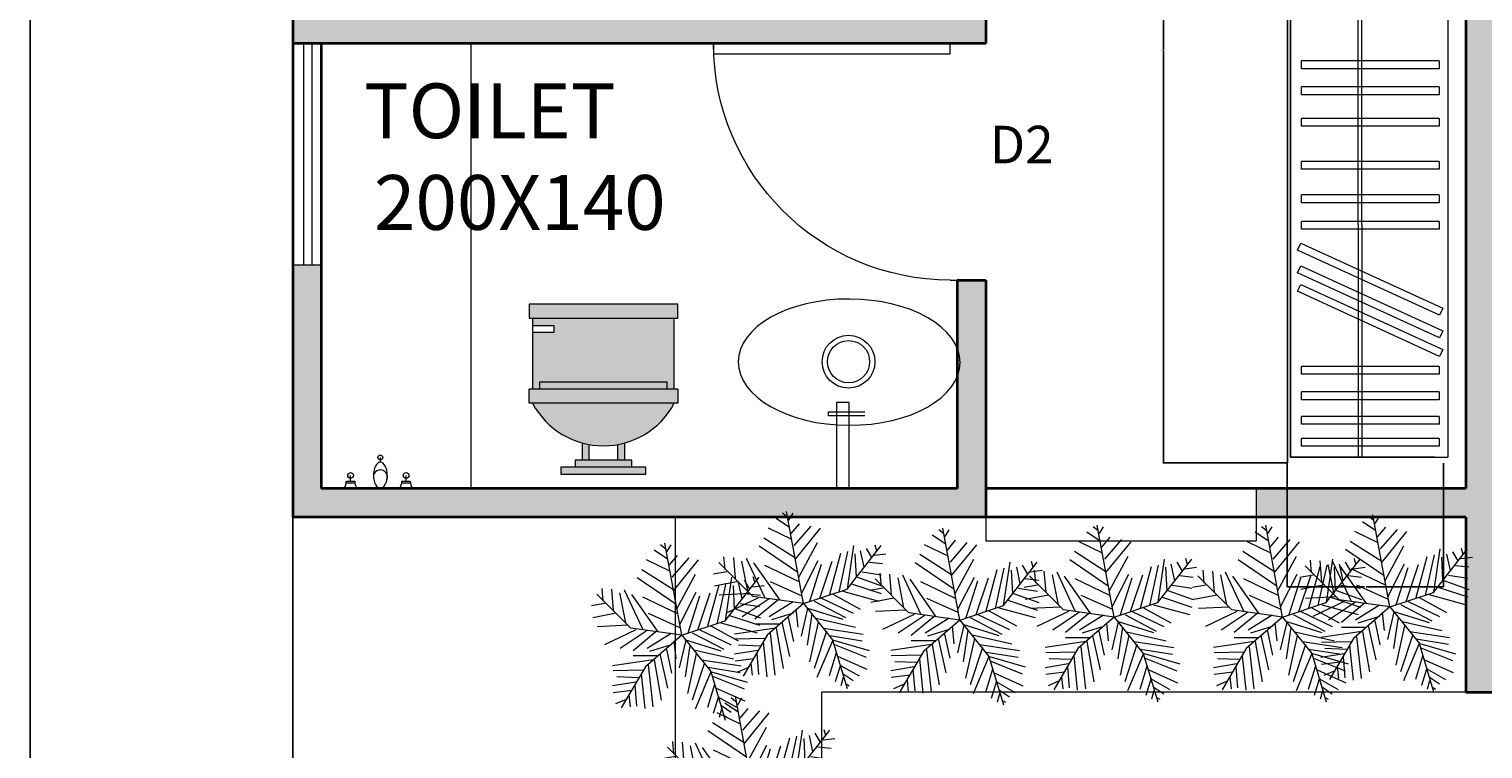
# Model space of a CAD drawing. Units: inches. Extents: x 192 to 1361, y -1362 to 367.
# Tile 2 of 23: x 192 to 649, y -987 to -761. Entities that reach past the tile are written whole.
import ezdxf

# ---------------------------------------------------------------- set-up
doc = ezdxf.new("R2010")
doc.units = ezdxf.units.IN
doc.header["$MEASUREMENT"] = 0
for name, color, linetype, lineweight in [('A-ANNO-DIMS', 2, 'Continuous', 18), ('A-AREA-IDEN', 7, 'Continuous', 18), ('A-DOOR', 4, 'Continuous', 18), ('A-FLOR', 8, 'Continuous', 18), ('A-FLOR-FIXT', 8, 'Continuous', 18), ('A-WALL-PATT', 250, 'Continuous', 13), ('closet', 32, 'Continuous', 18), ('lawn', 96, 'Continuous', 13), ('text', 7, 'Continuous', 18), ('walls', 7, 'Continuous', 35), ('windows', 4, 'Continuous', 18)]:
    doc.layers.add(name, color=color, linetype=linetype, lineweight=lineweight)
doc.layers.add('A-FLOR-FIXT-PATT', color=251, linetype='Continuous', lineweight=13, true_color=0x636466)
doc.styles.get("Standard").update_dxf_attribs({"font": 'arial.ttf'})
doc.dimstyles.get("Standard").update_dxf_attribs({"dimtxt": 0.18, "dimasz": 0.18, "dimexe": 0.18, "dimexo": 0.0625, "dimgap": 0.09, "dimtad": 0, "dimtih": 1, "dimtoh": 1, "dimzin": 0, "dimdsep": 46, "dimlunit": 3, "dimtxsty": 'Standard', "dimcen": 0.09, "dimadec": 0, "dimazin": 0, "dimtfac": 1, "dimtofl": 0, "dimtmove": 0, "dimatfit": 3, "dimfxl": 1, "dimtolj": 1, "dimtzin": 0, "dimarcsym": 0})

# ---------------------------------------------------------------- blocks, each defined once
blk = doc.blocks.new('*U2')
for p, q in [((0, 0), (0, -6)), ((40, 0), (40, -6))]:
    blk.add_line(p, q)
blk.add_lwpolyline([(0, 0), (0, 40), (1.75, 40), (1.75, 0)], close=True)
blk.add_arc((0, 0), 40, 0, 90)
blk = doc.blocks.new('*U4')
for p, q in [((-10.186, 53.64), (-13.084, 55.962)), ((0, 0), (-10.5, 57)), ((-9.099, 51.782), (-6.563, 55.962)), ((-7.288, 39.707), (-21.778, 46.673)), ((-8.737, 47.138), (-17.069, 52.711)), ((-7.65, 43.423), (-2.578, 49.46)), ((-5.839, 35.992), (4.667, 48.067)), ((-5.114, 27.632), (10.463, 46.673)), ((-5.114, 28.097), (-24.676, 40.636)), ((-2.941, 16.486), (8.652, 37.85)), ((44.153, 36.456), (45.239, 32.741)), ((-48.585, 21.131), (-49.309, 29.026)), ((-43.513, 28.561), (-42.427, 15.558)), ((-35.544, 28.097), (-24.314, 3.947)), ((-3.665, 19.273), (-27.574, 35.527)), ((16.259, 5.805), (23.142, 31.348)), ((22.055, 7.198), (27.489, 32.277)), ((27, 9), (48, 36)), ((27.127, 9.056), (31.112, 35.992)), ((31.836, 30.883), (32.561, 16.486)), ((35.096, 32.741), (37.27, 22.524)), ((38.719, 34.134), (41.979, 28.561)), ((43.791, 29.954), (51.036, 30.883)), ((-47.498, 19.737), (-55.83, 18.344)), ((-31.5, 4.5), (-52.5, 25.5)), ((-38.442, 26.239), (-34.819, 7.663)), ((-14.533, 2.09), (-30.834, 25.31)), ((-24.314, 23.917), (-2.941, 13.7)), ((-1.129, 6.734), (9.014, 26.704)), ((3.942, 1.625), (11.187, 24.381)), ((10.101, 3.483), (17.708, 26.239)), ((36.183, 19.737), (48.137, 17.88)), ((40.53, 25.775), (48.862, 24.846)), ((-40.615, 13.7), (-55.105, 10.913)), ((-20.691, 13.7), (-1.129, 4.876)), ((29.662, 12.307), (48.137, 6.269)), ((33.285, 16.486), (48.862, 10.913)), ((-33.37, 6.269), (-52.207, 5.34)), ((-28.299, 3.483), (-47.86, -5.805)), ((-21.416, 3.018), (-38.079, -8.128)), ((0, 0), (-31.5, 4.5)), ((-15.982, 2.09), (-30.11, -9.521)), ((0, 0), (-22.5, -19.5)), ((-6.563, 1.161), (-21.416, -8.128)), ((0, 0), (27, 9)), ((0, 0), (18, -22.5)), ((6.478, 1.625), (26.04, -8.592)), ((11.187, 3.483), (30.749, -5.805)), ((18.07, 5.805), (35.096, -3.483)), ((24.229, 7.663), (46.688, 1.625)), ((-6.563, -5.805), (-19.967, -9.985)), ((-9.461, -8.592), (-6.201, -23.453)), ((-4.752, -3.483), (-3.665, -14.629)), ((2.493, -3.019), (-1.491, -20.202)), ((1.769, -2.555), (24.229, -9.521)), ((5.029, -6.27), (2.131, -25.775)), ((-17.431, -15.094), (-42.789, -18.809)), ((-15.257, -12.772), (-30.11, -12.772)), ((-17.069, -15.094), (-12.721, -40.172)), ((-13.446, -11.378), (-8.737, -32.741)), ((9.014, -11.378), (3.58, -35.992)), ((14.085, -16.951), (6.478, -40.172)), ((7.565, -9.056), (32.198, -14.629)), ((12.274, -15.094), (36.907, -18.809)), ((-24.314, -21.596), (-42.427, -22.06)), ((-26.849, -26.24), (-40.253, -25.775)), ((-22.5, -19.5), (-37.5, -45)), ((-25.038, -23.918), (-22.865, -45.281)), ((-20.691, -18.345), (-17.793, -44.352)), ((18.07, -22.524), (8.289, -45.745)), ((16.259, -19.738), (36.183, -22.989)), ((18, -22.5), (27, -52.5)), ((18.433, -22.524), (40.53, -29.026)), ((19.157, -25.311), (38.719, -33.206)), ((-28.299, -29.026), (-42.789, -31.348)), ((-30.834, -34.135), (-42.427, -35.528)), ((-29.023, -30.884), (-27.936, -43.887)), ((20.244, -30.419), (15.897, -44.816)), ((21.331, -32.741), (39.081, -40.636)), ((-34.457, -39.708), (-40.978, -42.494)), ((-32.646, -36.921), (-31.921, -44.352)), ((22.78, -37.85), (19.519, -48.532)), ((22.78, -38.314), (34.372, -44.816)), ((24.591, -43.423), (30.749, -47.603)), ((24.591, -45.745), (23.142, -50.854)), ((26.764, -49.925), (28.213, -50.854))]:
    blk.add_line(p, q)
blk = doc.blocks.new('closet')
at = {"layer": 'closet'}
for p, q in [((-0.71, -5.58), (5.59, 8.19)), ((-0.23, 7.39), (-0.23, -6.57)), ((6.27, 7.88), (-0.04, -5.89)), ((5.59, 8.19), (6.27, 7.88)), ((7.92, 7.84), (8.68, 7.84)), ((7.92, 7.84), (7.92, -5.51)), ((8.68, 7.84), (8.68, -5.51)), ((10.44, 7.84), (11.2, 7.84)), ((10.44, 7.84), (10.44, -5.51)), ((11.2, 7.84), (11.2, -5.51)), ((12.45, 7.84), (13.21, 7.84)), ((12.45, 7.84), (12.45, -5.51)), ((13.21, 7.84), (13.21, -5.51)), ((14.71, 7.84), (15.47, 7.84)), ((14.71, 7.84), (14.71, -5.51)), ((15.47, 7.84), (15.47, -5.51)), ((17.44, 7.75), (18.17, 7.93)), ((17.44, 7.75), (20.73, -5.2)), ((18.17, 7.93), (21.46, -5.01)), ((23.92, 7.84), (22.75, -5.46)), ((24.67, 7.78), (23.51, -5.53)), ((23.92, 7.84), (24.67, 7.78)), ((26.09, 8.25), (26.09, -5.1)), ((26.84, 8.25), (26.84, -5.1)), ((29.49, 7.29), (32.64, -5.69)), ((30.22, 7.46), (33.37, -5.51)), ((35.23, 7.84), (35.23, -5.51)), ((35.99, 7.84), (35.99, -5.51)), ((40.33, 7.84), (40.33, -5.51)), ((41.08, 7.84), (41.08, -5.51)), ((42.85, 7.84), (42.85, -5.51)), ((43.61, 7.84), (43.61, -5.51)), ((45.9, 7.84), (45.9, -5.51)), ((46.65, 7.84), (46.65, -5.51)), ((50.07, 7.84), (50.07, -5.51)), ((50.82, 7.84), (50.82, -5.51)), ((53.32, 7.84), (53.32, -5.51)), ((54.08, 7.84), (54.08, -5.51)), ((55.9, 7.84), (55.9, -5.51)), ((56.65, 7.84), (56.65, -5.51)), ((57.99, -5.58), (64.3, 8.19)), ((64.97, 7.88), (58.67, -5.89)), ((60.19, -5.58), (66.49, 8.19)), ((67.17, 7.88), (60.87, -5.89)), ((62, -5.58), (68.3, 8.19)), ((68.98, 7.88), (62.67, -5.89)), ((69.96, 7.84), (69.96, -5.51)), ((70.72, 7.84), (70.72, -5.51)), ((72.43, 7.84), (72.43, -5.51)), ((73.19, 7.84), (73.19, -5.51)), ((74.82, 7.84), (74.82, -5.51)), ((75.57, 7.84), (75.57, -5.51)), ((76.94, 7.84), (76.94, -5.51)), ((77.69, 7.84), (77.69, -5.51)), ((56.23, 0.33), (0, 0.33)), ((56.2, 0), (0, 0)), ((56.2, 0), (78.76, 0)), ((56.23, 0.33), (78.76, 0.33)), ((-0.04, -5.89), (-0.71, -5.58)), ((21.46, -5.01), (20.73, -5.2)), ((23.51, -5.53), (22.75, -5.46)), ((33.37, -5.51), (32.64, -5.69)), ((35.99, -5.51), (35.23, -5.51)), ((41.08, -5.51), (40.33, -5.51)), ((43.61, -5.51), (42.85, -5.51)), ((46.65, -5.51), (45.9, -5.51)), ((50.82, -5.51), (50.07, -5.51)), ((54.08, -5.51), (53.32, -5.51)), ((56.65, -5.51), (55.9, -5.51)), ((58.67, -5.89), (57.99, -5.58)), ((60.87, -5.89), (60.19, -5.58)), ((62.67, -5.89), (62, -5.58)), ((70.72, -5.51), (69.96, -5.51)), ((73.19, -5.51), (72.43, -5.51)), ((75.57, -5.51), (74.82, -5.51)), ((77.69, -5.51), (76.94, -5.51))]:
    blk.add_line(p, q, dxfattribs=at)
blk = doc.blocks.new('rotated closet')
at = {"layer": 'closet'}
for p, q in [((26.32, 0.86), (27.07, 0.86)), ((29.72, -0.11), (30.45, 0.07)), ((35.46, 0.45), (36.22, 0.45)), ((40.56, 0.45), (41.31, 0.45)), ((43.08, 0.45), (43.84, 0.45)), ((46.13, 0.45), (46.88, 0.45)), ((50.3, 0.45), (51.05, 0.45)), ((53.56, 0.45), (54.31, 0.45)), ((56.13, 0.45), (56.88, 0.45)), ((64.53, 0.8), (65.2, 0.49)), ((66.72, 0.8), (67.4, 0.49)), ((68.53, 0.8), (69.21, 0.49)), ((70.19, 0.45), (70.95, 0.45)), ((72.66, 0.45), (73.42, 0.45)), ((75.05, 0.45), (75.81, 0.45)), ((77.17, 0.45), (77.92, 0.45)), ((78.99, 0), (78.99, -13.96)), ((0, -13.96), (78.99, -13.96)), ((8.91, -12.91), (8.15, -12.91)), ((11.43, -12.91), (10.67, -12.91)), ((13.44, -12.91), (12.68, -12.91)), ((15.7, -12.91), (14.94, -12.91)), ((-0.46, -14.27), (79.54, -14.27))]:
    blk.add_line(p, q, dxfattribs=at)
blk.add_blockref('closet', (0.23, -7.39), dxfattribs=at)
blk = doc.blocks.new('*U18')
for p, q in [((-10, 22), (-10, 12)), ((-10, 21), (-7, 21)), ((-7, 21), (-7, 20)), ((10, 12), (10, 22)), ((-7, 20), (-10, 20)), ((9, 13), (-9, 13)), ((-9, 13), (-9, 12)), ((9, 12), (9, 13)), ((10.5, 12), (-10.5, 12)), ((-10.5, 10), (-10.5, 12)), ((10.5, 12), (10.5, 10)), ((10.5, 10), (-10.5, 10)), ((-3, 4.4065), (-3, 2)), ((-2, 2), (-2, 4.1658)), ((2, 4.1658), (2, 2)), ((3, 2), (3, 4.4065)), ((4, 2), (-4, 2)), ((-4, 2), (-4, 1)), ((4, 1), (4, 2))]:
    blk.add_line(p, q)
for points in [[(10.5, 22), (10.5, 24), (-10.5, 24), (-10.5, 22)], [(6, 0), (6, 1), (-6, 1), (-6, 0)]]:
    blk.add_lwpolyline(points, close=True)
blk.add_arc((0, 15.3333), 11.3333, 208.0725, 331.9275)
blk = doc.blocks.new('BASIN-OVAL-WITH-TAP')
for p, q in [((-0.13, -12.72), (-4, -12.74)), ((-4, -12.74), (-4, -39.43)), ((-0.13, -12.72), (-0.13, -39.43)), ((-6.48, -15.66), (4.91, -15.61)), ((-6.47, -16.92), (-6.48, -15.66)), ((4.94, -16.86), (-6.47, -16.92))]:
    blk.add_line(p, q)
for radius in [8.31, 6.64]:
    blk.add_circle((-0.19, 0.14), radius)
at = {"extrusion": (0, 0, -1)}
blk.add_ellipse((0, 0), major_axis=(-34.9, 0.1), ratio=0.56899, dxfattribs=at)
blk = doc.blocks.new('BATH-MIXER-TWIN-HANDLE')
for p, q in [((0, 4.11), (0, 5.63)), ((-10.73, -2.32), (-8.02, -2.36)), ((-10.7, -1.84), (-8.05, -1.84)), ((-9.38, -1.84), (-9.38, -0.03)), ((6.73, -2.31), (9.44, -2.32)), ((6.76, -1.84), (9.41, -1.84)), ((8.08, -1.84), (8.08, -0.03))]:
    blk.add_line(p, q)
for centre, radius in [((0, 5.63), 0.761), ((-9.38, -0.03), 0.904), ((8.08, -0.03), 0.904)]:
    blk.add_circle(centre, radius)
for centre, radius, start, end in [((0, -0.5), 2.23, 336.3452, 166.942), ((-14.82, -1.84), 4.11, 326.5495, 0), ((-3.94, -1.84), 4.11, 180, 213.4505), ((2.65, -1.84), 4.11, 326.5495, 0), ((13.52, -1.84), 4.11, 180, 213.4505)]:
    blk.add_arc(centre, radius, start, end)
at = {"extrusion": (0, 0, -1)}
blk.add_ellipse((0, 0), major_axis=(0, -4.11), ratio=0.528671, dxfattribs=at)
blk = doc.blocks.new('*D31')
at = {"layer": 'A-ANNO-DIMS', "color": 0, "lineweight": -2, "transparency": 16777216}
for p, q in [((587.7, -637.86), (548.65, -637.86)), ((548.83, -638.04), (548.83, -767.46)), ((548.83, -897.24), (548.83, -767.83)), ((587.7, -897.42), (548.65, -897.42))]:
    blk.add_line(p, q, dxfattribs=at)
at = {"layer": 'A-ANNO-DIMS', "color": 0, "transparency": 16777216}
for points in [[(548.8, -638.04), (548.86, -638.04), (548.83, -637.86)], [(548.8, -897.24), (548.86, -897.24), (548.83, -897.42)]]:
    blk.add_solid(points, dxfattribs=at)
at = {"layer": 'Defpoints', "color": 0, "transparency": 16777216}
for p in [(587.76, -637.86), (548.83, -897.42), (587.76, -897.42)]:
    blk.add_point(p, dxfattribs=at)
at = {"layer": 'A-ANNO-DIMS', "color": 0, "transparency": 16777216, "insert": (548.83, -767.64), "char_height": 0.18, "attachment_point": 5}
blk.add_mtext('\\A1;WARDROBE 260', dxfattribs=at)
blk = doc.blocks.new('*D32')
at = {"layer": 'A-ANNO-DIMS', "color": 0, "lineweight": -2, "transparency": 16777216}
for p, q in [((587.76, -897.48), (587.76, -936.54)), ((636.85, -897.48), (636.85, -936.54)), ((587.94, -936.36), (612.08, -936.36)), ((636.67, -936.36), (612.53, -936.36))]:
    blk.add_line(p, q, dxfattribs=at)
at = {"layer": 'A-ANNO-DIMS', "color": 0, "transparency": 16777216}
for points in [[(587.94, -936.33), (587.94, -936.39), (587.76, -936.36)], [(636.67, -936.33), (636.67, -936.39), (636.85, -936.36)]]:
    blk.add_solid(points, dxfattribs=at)
at = {"layer": 'Defpoints', "color": 0, "transparency": 16777216}
for p in [(587.76, -897.42), (636.85, -897.42), (636.85, -936.36)]:
    blk.add_point(p, dxfattribs=at)
at = {"layer": 'A-ANNO-DIMS', "color": 0, "transparency": 16777216, "insert": (612.31, -936.36), "char_height": 0.18, "attachment_point": 5}
blk.add_mtext('\\A1;49', dxfattribs=at)
blk = doc.blocks.new('*D47')
at = {"layer": 'A-ANNO-DIMS', "color": 0, "lineweight": -2, "transparency": 16777216}
for p, q in [((1273.57, -782.95), (1273.57, -1200.05)), ((274.89, -914.5), (274.89, -1200.05)), ((275.07, -1199.87), (773.84, -1199.87)), ((1273.39, -1199.87), (774.62, -1199.87))]:
    blk.add_line(p, q, dxfattribs=at)
at = {"layer": 'A-ANNO-DIMS', "color": 0, "transparency": 16777216}
for points in [[(275.07, -1199.84), (275.07, -1199.9), (274.89, -1199.87)], [(1273.39, -1199.84), (1273.39, -1199.9), (1273.57, -1199.87)]]:
    blk.add_solid(points, dxfattribs=at)
at = {"layer": 'Defpoints', "color": 0, "transparency": 16777216}
for p in [(1273.57, -782.89), (274.89, -914.44), (1273.57, -1199.87)]:
    blk.add_point(p, dxfattribs=at)
at = {"layer": 'A-ANNO-DIMS', "color": 0, "transparency": 16777216, "insert": (774.23, -1199.87), "char_height": 0.18, "attachment_point": 5}
blk.add_mtext('\\A1;998.7', dxfattribs=at)
blk = doc.blocks.new('*D48')
at = {"layer": 'A-ANNO-DIMS', "color": 0, "lineweight": -2, "transparency": 16777216}
for p, q in [((325.63, 258.53), (192.16, 258.53)), ((192.34, 258.35), (192.34, -429.22)), ((192.34, -1117.14), (192.34, -429.58)), ((395.21, -1117.32), (192.16, -1117.32))]:
    blk.add_line(p, q, dxfattribs=at)
at = {"layer": 'A-ANNO-DIMS', "color": 0, "transparency": 16777216}
for points in [[(192.31, 258.35), (192.37, 258.35), (192.34, 258.53)], [(192.31, -1117.14), (192.37, -1117.14), (192.34, -1117.32)]]:
    blk.add_solid(points, dxfattribs=at)
at = {"layer": 'Defpoints', "color": 0, "transparency": 16777216}
for p in [(325.7, 258.53), (192.34, -1117.32), (395.28, -1117.32)]:
    blk.add_point(p, dxfattribs=at)
at = {"layer": 'A-ANNO-DIMS', "color": 0, "transparency": 16777216, "insert": (192.34, -429.4), "char_height": 0.18, "attachment_point": 5}
blk.add_mtext('\\A1;1375.9', dxfattribs=at)

msp = doc.modelspace()

# ---------------------------------------------------------------- hatches: boundary and pattern name
at = {"layer": 'A-FLOR-FIXT-PATT'}
h = msp.add_hatch(color=256, dxfattribs=at)
h.dxf.hatch_style = 1
h.paths.add_polyline_path([(394.9366, -851.9167), (350.3431, -851.9167), (350.3431, -854.1464), (357.0321, -854.1464), (357.0321, -856.3761), (350.3431, -856.3761), (350.3431, -874.2135), (352.5728, -874.2135), (352.5728, -871.9838), (392.7069, -871.9838), (392.7069, -874.2135), (394.9366, -874.2135)])
h.paths.add_polyline_path([(396.0514, -847.4574), (349.2282, -847.4574), (349.2282, -851.9167), (396.0514, -851.9167)])
h.paths.add_polyline_path([(396.0514, -874.2135), (349.2282, -874.2135), (349.2282, -878.6728), (396.0514, -878.6728)])
h.paths.add_polyline_path([(392.7069, -871.9838), (352.5728, -871.9838), (352.5728, -874.2135), (392.7069, -874.2135)], flags=17)
h.paths.add_polyline_path([(394.9366, -878.6728), (350.343, -878.6728, 0.60000216)])
h.paths.add_polyline_path([(368.1805, -891.6544, -0.0226287), (365.9508, -891.1496), (365.9508, -896.5102), (368.1805, -896.5102)])
h.paths.add_polyline_path([(379.3288, -891.1496, -0.0226287), (377.0992, -891.6544), (377.0992, -896.5102), (379.3288, -896.5102)])
h.paths.add_polyline_path([(381.5585, -896.5102), (363.7211, -896.5102), (363.7211, -898.7399), (381.5585, -898.7399)])
h.paths.add_polyline_path([(386.0179, -898.7399), (359.2618, -898.7399), (359.2618, -900.9696), (386.0179, -900.9696)])
at = {"layer": 'A-WALL-PATT'}
h = msp.add_hatch(color=256, dxfattribs=at)
h.dxf.hatch_style = 1
h.paths.add_polyline_path([(309.5452, 191.102), (300.5452, 191.102), (300.5452, -126.898), (309.5452, -126.898), (309.5452, -117.898)])
h.paths.add_polyline_path([(420.798, 191.102), (337.3229, 191.102), (337.3229, 182.102), (420.798, 182.102)])
h.paths.add_polyline_path([(518.5452, 182.102), (625.4022, 182.102), (625.4022, 191.102), (509.5452, 191.102), (509.5452, 114.3262), (518.5452, 114.3262)])
h.paths.add_polyline_path([(842.5452, 191.102), (763.4438, 191.102), (763.4438, 182.102), (833.5452, 182.102), (833.5452, 161.1615), (836.8088, 161.1615), (842.5452, 161.1615)])
h.paths.add_polyline_path([(842.5452, -16.5675), (833.5452, -16.5675), (833.5452, -60.4996), (784.8041, -60.4996), (784.8041, -354.6796), (793.8041, -354.6796), (793.8041, -69.4996), (1094.1252, -69.4996), (1094.1252, -60.4996), (842.5452, -60.4996)])
h.paths.add_polyline_path([(518.5452, 36.602), (509.5452, 36.602), (509.5452, -117.898), (420.2204, -117.898), (420.2204, -126.898), (518.5452, -126.898)])
h.paths.add_polyline_path([(474.8041, -377.0384), (465.8041, -377.0384), (465.8041, -381.5384), (465.8041, -450.898), (537.5717, -450.898), (537.5717, -441.898), (474.8041, -441.898)])
h.paths.add_polyline_path([(1162.8041, -380.6763), (1204.3001, -380.6763), (1204.3001, -375.6763), (1195.1471, -375.6763), (1153.8041, -375.6763), (1153.8041, -448.4996), (856.5691, -448.4996), (856.5691, -457.4996), (1162.8041, -457.4996)])
h.paths.add_polyline_path([(1162.8041, -525.128), (1153.8041, -525.128), (1153.8041, -597.4996), (1162.8041, -597.4996)], flags=17)
h.paths.add_polyline_path([(1162.8041, -60.4996), (1153.8041, -60.4996), (1153.8041, -69.4996), (1153.8041, -177.4733), (1205.8889, -177.4733), (1205.8889, -172.4733), (1162.8041, -172.4733)])
h.paths.add_polyline_path([(980.5799, -525.686), (971.5799, -525.686), (971.5799, -597.4996), (980.5799, -597.4996)], flags=17)
h.paths.add_polyline_path([(856.5691, -448.4996), (798.7542, -448.4996), (784.8041, -448.4996), (784.8041, -457.4996), (847.5691, -457.4996), (847.5691, -597.4996), (784.8041, -597.4996), (784.8041, -606.4996), (1273.5658, -606.4996), (1273.5658, -597.4996), (856.5691, -597.4996)])
h.paths.add_polyline_path([(1273.5658, -773.892), (1099.8366, -773.892), (1099.8366, -851.9362), (1108.8366, -851.9362), (1108.8366, -782.892), (1273.5658, -782.892)])
h.paths.add_polyline_path([(1108.8366, -982.9214), (1099.8366, -982.9214), (1099.8366, -1067.6246), (1037.7563, -1067.6246), (1037.7563, -1076.6246), (1108.8366, -1076.6246)])
h.paths.add_polyline_path([(835.078, -1067.6246), (758.8458, -1067.6246), (758.8458, -940.2324), (749.8458, -940.2324), (749.8458, -963.172), (749.8458, -970.4644), (749.8458, -1076.6246), (835.078, -1076.6246)])
h.paths.add_polyline_path([(450.307, -1066.9838), (441.307, -1066.9838), (441.307, -1076.6246), (450.307, -1076.6246)])
h.paths.add_polyline_path([(492.8925, -756.4415), (274.8925, -756.4415), (274.8925, -765.4415), (492.8925, -765.4415)])
h.paths.add_polyline_path([(283.8925, -835.2244), (274.8925, -835.2244), (274.8925, -914.4415), (492.8925, -914.4415), (492.8925, -839.9415), (483.8925, -839.9415), (483.8925, -905.4415), (283.8925, -905.4415)])
h.paths.add_polyline_path([(283.8925, -441.898), (283.8925, -375.4296), (281.6021, -375.4296), (281.6021, -399.4121), (274.8925, -399.4121), (274.8925, -441.898), (274.8925, -684.5089), (283.8925, -684.5089)])
h = msp.add_hatch(color=256, dxfattribs=at)
h.dxf.hatch_style = 1
h.paths.add_polyline_path([(652.8925, -441.898), (643.8925, -441.898), (643.8925, -457.8461), (643.8925, -564.167), (643.8925, -905.4415), (578.0245, -905.4415), (578.0245, -914.4415), (643.8925, -914.4415), (643.8925, -969.5484), (652.6138, -969.5484), (652.6138, -963.172), (652.6138, -914.556)])
h.paths.add_polyline_path([(509.5452, 191.102), (504.3983, 191.102), (504.3983, 182.102), (509.5452, 182.102)])

# ---------------------------------------------------------------- linework, layer by layer
at = {"layer": 'A-FLOR'}
for p, q in [((395.2768, -1076.6246), (395.2768, -914.4415)), ((441.307, -1076.6246), (441.307, -969.5484)), ((643.8925, -969.5484), (441.307, -969.5484))]:
    msp.add_line(p, q, dxfattribs=at)
at = {"layer": 'A-FLOR-FIXT'}
msp.add_line((331.0404, -905.4415), (331.0404, -765.4415), dxfattribs=at)
at = {"layer": 'closet'}
for p, q in [((587.7625, -637.9412), (587.7625, -897.4218)), ((588.7836, -895.6222), (588.7836, -639.4217)), ((638.256, -639.4217), (638.256, -895.6222)), ((588.7836, -895.6222), (638.256, -895.6222)), ((638.256, -895.6222), (638.256, -895.6222))]:
    msp.add_line(p, q, dxfattribs=at)
at = {"layer": 'walls'}
for p, q in [((274.8925, -441.898), (274.8925, -914.4415)), ((643.8925, -441.898), (643.8925, -905.4415)), ((492.8925, -756.4415), (492.8925, -765.4415)), ((492.8925, -765.4415), (274.8925, -765.4415)), ((283.8925, -765.4415), (283.8925, -905.4415)), ((483.8925, -839.9008), (483.8925, -905.4415)), ((483.8925, -839.9415), (492.8925, -839.9415)), ((492.8925, -839.9008), (492.8925, -914.4415)), ((483.8925, -905.4415), (283.8925, -905.4415)), ((643.8925, -905.4415), (492.8925, -905.4415)), ((643.8925, -914.4415), (274.8925, -914.4415)), ((643.8925, -914.4415), (643.8925, -969.5484)), ((643.8925, -969.5484), (652.8925, -969.5484))]:
    msp.add_line(p, q, dxfattribs=at)
at = {"layer": 'windows'}
for p, q in [((283.8925, -765.4415), (274.8925, -765.4415)), ((283.8925, -765.4415), (274.8925, -765.4415)), ((278.2403, -765.4415), (278.2403, -835.2244)), ((280.9699, -835.2244), (280.9699, -765.4415)), ((283.8925, -835.2244), (274.8925, -835.2244)), ((578.0245, -921.9715), (578.0245, -905.4415)), ((492.8925, -914.4415), (492.8925, -921.9715)), ((492.8925, -921.9715), (578.0245, -921.9715))]:
    msp.add_line(p, q, dxfattribs=at)

# ---------------------------------------------------------------- block references
at = {"layer": 'A-DOOR', "xscale": -1.861483602217143, "yscale": 1.861483602217143, "zscale": 1.861483602217143, "rotation": 90}
msp.add_blockref('*U2', (481.7236, -765.4415), dxfattribs=at)
at = {"layer": 'A-FLOR-FIXT'}
for name, p in [('BASIN-OVAL-WITH-TAP', (449.9329, -865.7223)), ('BATH-MIXER-TWIN-HANDLE', (302.4694, -901.3344))]:
    msp.add_blockref(name, p, dxfattribs=at)
at = {"layer": 'A-FLOR-FIXT', "xscale": 2.229674534520691, "yscale": 2.229674534520691, "zscale": 2.229674534520691}
msp.add_blockref('*U18', (372.6398, -900.9696), dxfattribs=at)
at = {"layer": 'closet', "xscale": 3.243507334136714, "yscale": 3.243507334136714, "zscale": 3.243507334136714, "rotation": 269.9999999992008}
msp.add_blockref('rotated closet', (634.0617, -639.4217), dxfattribs=at)
at = {"layer": 'lawn', "xscale": 0.5078671948952364, "yscale": 0.5078671948952364, "zscale": 0.5078671948952364}
for p in [(435.6007, -941.6936), (620.0437, -942.7451), (484.7335, -946.8825), (533.3158, -945.9389), (586.2918, -945.9389), (397.2462, -951.6555), (419.4939, -999.7959)]:
    msp.add_blockref('*U4', p, dxfattribs=at)

# ---------------------------------------------------------------- texts
at = {"layer": 'A-AREA-IDEN'}
for s, p in [('TOILET', (297.3013, -795.2734)), ('200X140', (300.4343, -824.1029))]:
    msp.add_text(s, height=17.23824, dxfattribs=at).set_placement(p)
at = {"layer": 'text'}
msp.add_text('D2', height=11.81288, dxfattribs=at).set_placement((494.2043, -803.1855))

# ---------------------------------------------------------------- dimensions: what is measured, and where the dimension line sits
at = {"layer": 'A-ANNO-DIMS'}
dim = msp.add_linear_dim(base=(192.3425, -1117.3227), p1=(325.6957, 258.5286), p2=(395.2768, -1117.3227), angle=90, dimstyle='Standard', override={"dimdec": 1, "dimlfac": 1, "dimrnd": 0, "dimzin": 0, "dimdsep": 46, "dimlunit": 2}, dxfattribs=at)
dim.commit()
dim.dimension.update_dxf_attribs({"geometry": '*D48', "text_midpoint": (192.3425, -429.3971)})
dim = msp.add_linear_dim(base=(548.8289, -897.4218), p1=(587.7625, -637.8641), p2=(587.7625, -897.4218), angle=270, text='WARDROBE <>', dimstyle='Standard', override={"dimdec": 0, "dimlfac": 1, "dimrnd": 0, "dimzin": 0, "dimdsep": 46, "dimlunit": 2}, dxfattribs=at)
dim.commit()
dim.dimension.update_dxf_attribs({"geometry": '*D31', "text_midpoint": (548.8289, -767.6429)})
for base, p1, p2, override, picture, middle in [((1273.5658, -1199.8727), (274.8925, -914.4415), (1273.5658, -782.892), {"dimdec": 1, "dimlfac": 1, "dimrnd": 0, "dimzin": 0, "dimdsep": 46, "dimlunit": 2}, '*D47', (774.2292, -1199.8727)), ((636.8504, -936.3554), (587.7625, -897.4218), (636.8504, -897.4218), {"dimdec": 0, "dimlfac": 1, "dimrnd": 0, "dimzin": 0, "dimdsep": 46, "dimlunit": 2}, '*D32', (612.3065, -936.3554))]:
    dim = msp.add_linear_dim(base=base, p1=p1, p2=p2, dimstyle='Standard', override=override, dxfattribs=at)
    dim.commit()
    dim.dimension.update_dxf_attribs({"geometry": picture, "text_midpoint": middle})

doc.saveas('drawing.dxf')
